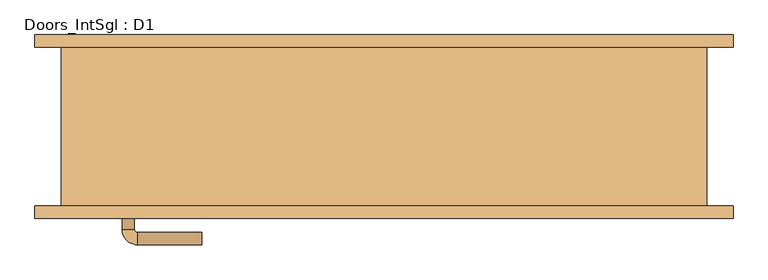
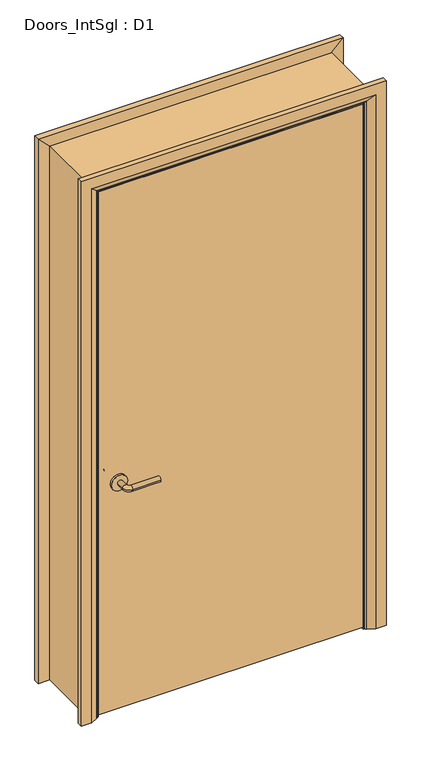
"""IFC4 building model written with IfcOpenShell, lengths in millimetres: door geometry, Doors_IntSgl : D1."""

from ifc_helpers import new_model, si_unit, point, frame, frame_2d, origin, place, context, project, spatial, polyline, circle_curve, ellipse_curve, trimmed, segment, composite_curve, outline, extrude, faceted_brep, source, transform, mapped, element, save
from ifc_brep_helpers import plane_surface, cylinder_surface, revolved_surface, advanced_brep


def doors_intsgl_d1_0a18db40(model_context):
    return source(origin(), model_context, "Body", "SolidModel", [
        advanced_brep(
        [(-426.4, -83.54, 900.0), (-406.4, -83.54, 900.0), (-426.4, -53.54, 900.0), (-406.4, -53.54, 900.0), (-401.4, -48.54, 900.0), (-401.4, -28.54, 900.0), (-296.4, -28.54, 900.0), (-296.4, -48.54, 900.0)],
        [
            (0, 1, circle_curve(frame((-416.4, -83.54, 900.0), z_axis=(0.0, -1.0, 0.0), x_axis=(1.0, 0.0, 0.0)), 10.0)),
            (1, 0, circle_curve(frame((-416.4, -83.54, 900.0), z_axis=(0.0, -1.0, 0.0), x_axis=(1.0, 0.0, 0.0)), 10.0)),
            (0, 2),
            (2, 3, circle_curve(frame((-416.4, -53.54, 900.0), z_axis=(0.0, -1.0, 0.0), x_axis=(1.0, 0.0, 0.0)), 10.0)),
            (3, 1),
            (3, 2, circle_curve(frame((-416.4, -53.54, 900.0), z_axis=(0.0, -1.0, 0.0), x_axis=(1.0, 0.0, 0.0)), 10.0)),
            (4, 3, circle_curve(frame((-401.4, -53.54, 900.0), z_axis=(0.0, 0.0, 1.0), x_axis=(-1.0, 0.0, 0.0)), 5.0)),
            (2, 5, circle_curve(frame((-401.4, -53.54, 900.0), z_axis=(0.0, 0.0, -1.0), x_axis=(-1.0, 0.0, 0.0)), 25.0)),
            (5, 4, circle_curve(frame((-401.4, -38.54, 900.0), z_axis=(-1.0, 0.0, 0.0), x_axis=(0.0, -1.0, 0.0)), 10.0)),
            (4, 5, circle_curve(frame((-401.4, -38.54, 900.0), z_axis=(-1.0, 0.0, 0.0), x_axis=(0.0, -1.0, 0.0)), 10.0)),
            (6, 7, circle_curve(frame((-296.4, -38.54, 900.0), z_axis=(1.0, 0.0, 0.0), x_axis=(0.0, -1.0, 0.0)), 10.0)),
            (7, 6, circle_curve(frame((-296.4, -38.54, 900.0), z_axis=(1.0, 0.0, 0.0), x_axis=(0.0, -1.0, 0.0)), 10.0)),
            (5, 6),
            (7, 4),
        ],
        [
            plane_surface(frame((-416.4, -83.54, 900.0), z_axis=(0.0, -1.0, 0.0), x_axis=(0.0, 0.0, 1.0))),
            cylinder_surface(frame((-416.4, -83.54, 900.0), z_axis=(0.0, -1.0, 0.0), x_axis=(1.0, 0.0, 0.0)), 10.0),
            revolved_surface(trimmed(ellipse_curve(frame((-416.4, -53.54, 900.0), z_axis=(0.0, -1.0, 0.0), x_axis=(1.0, 0.0, 0.0)), 10.0, 10.0), [point((-426.4, -53.54, 900.0))], [point((-406.4, -53.54, 900.0))], True, "CARTESIAN"), (-401.4, -53.54, 900.0), (0.0, 0.0, -1.0)),
            revolved_surface(trimmed(ellipse_curve(frame((-416.4, -53.54, 900.0), z_axis=(0.0, -1.0, 0.0), x_axis=(1.0, 0.0, 0.0)), 10.0, 10.0), [point((-406.4, -53.54, 900.0))], [point((-426.4, -53.54, 900.0))], True, "CARTESIAN"), (-401.4, -53.54, 900.0), (0.0, 0.0, -1.0)),
            plane_surface(frame((-296.4, -38.54, 900.0), z_axis=(1.0, 0.0, 0.0), x_axis=(0.0, 0.0, 1.0))),
            cylinder_surface(frame((-401.4, -38.54, 900.0), z_axis=(-1.0, 0.0, 0.0), x_axis=(0.0, -1.0, 0.0)), 10.0),
        ],
        [
            (0, [[1, 2]]),
            (1, [[-1, 3, 4, 5]]),
            (1, [[-2, -5, 6, -3]]),
            (2, [[7, -4, 8, 9]]),
            (3, [[-8, -6, -7, 10]]),
            (4, [[11, 12]]),
            (5, [[-9, 13, -12, 14]]),
            (5, [[-10, -14, -11, -13]]),
        ],
    ),
        extrude(outline(composite_curve([segment(trimmed(circle_curve(frame_2d((900.0, -418.9)), 30.0), [point((900.0, -448.9))], [point((900.0, -388.9))], False, "CARTESIAN"), True, "CONTINUOUS"), segment(trimmed(circle_curve(frame_2d((900.0, -418.9)), 30.0), [point((900.0, -388.9))], [point((900.0, -448.9))], False, "CARTESIAN"), True, "CONTINUOUS")], self_intersect=False)), frame((0.0, -91.54, 0.0), z_axis=(0.0, 1.0, 0.0), x_axis=(0.0, 0.0, 1.0)), (0.0, 0.0, 1.0), 8.0),
        advanced_brep(
        [(-426.4, -137.54, 900.0), (-406.4, -137.54, 900.0), (-406.4, -167.54, 900.0), (-426.4, -167.54, 900.0), (-401.4, -172.54, 900.0), (-401.4, -192.54, 900.0), (-296.4, -192.54, 900.0), (-296.4, -172.54, 900.0)],
        [
            (0, 1, circle_curve(frame((-416.4, -137.54, 900.0), z_axis=(0.0, 1.0, 0.0), x_axis=(1.0, 0.0, 0.0)), 10.0)),
            (1, 0, circle_curve(frame((-416.4, -137.54, 900.0), z_axis=(0.0, 1.0, 0.0), x_axis=(1.0, 0.0, 0.0)), 10.0)),
            (1, 2),
            (2, 3, circle_curve(frame((-416.4, -167.54, 900.0), z_axis=(0.0, 1.0, 0.0), x_axis=(1.0, 0.0, 0.0)), 10.0)),
            (3, 0),
            (3, 2, circle_curve(frame((-416.4, -167.54, 900.0), z_axis=(0.0, 1.0, 0.0), x_axis=(1.0, 0.0, 0.0)), 10.0)),
            (4, 5, circle_curve(frame((-401.4, -182.54, 900.0), z_axis=(-1.0, 0.0, 0.0), x_axis=(0.0, 1.0, 0.0)), 10.0)),
            (5, 3, circle_curve(frame((-401.4, -167.54, 900.0), z_axis=(0.0, 0.0, -1.0), x_axis=(-1.0, 0.0, 0.0)), 25.0)),
            (2, 4, circle_curve(frame((-401.4, -167.54, 900.0), z_axis=(0.0, 0.0, 1.0), x_axis=(-1.0, 0.0, 0.0)), 5.0)),
            (5, 4, circle_curve(frame((-401.4, -182.54, 900.0), z_axis=(-1.0, 0.0, 0.0), x_axis=(0.0, 1.0, 0.0)), 10.0)),
            (6, 7, circle_curve(frame((-296.4, -182.54, 900.0), z_axis=(1.0, 0.0, 0.0), x_axis=(0.0, 1.0, 0.0)), 10.0)),
            (7, 6, circle_curve(frame((-296.4, -182.54, 900.0), z_axis=(1.0, 0.0, 0.0), x_axis=(0.0, 1.0, 0.0)), 10.0)),
            (4, 7),
            (6, 5),
        ],
        [
            plane_surface(frame((-416.4, -137.54, 900.0), z_axis=(0.0, 1.0, 0.0), x_axis=(0.0, 0.0, 1.0))),
            cylinder_surface(frame((-416.4, -137.54, 900.0), z_axis=(0.0, 1.0, 0.0), x_axis=(1.0, 0.0, 0.0)), 10.0),
            revolved_surface(trimmed(ellipse_curve(frame((-416.4, -167.54, 900.0), z_axis=(0.0, -1.0, 0.0), x_axis=(1.0, 0.0, 0.0)), 10.0, 10.0), [point((-426.4, -167.54, 900.0))], [point((-406.4, -167.54, 900.0))], True, "CARTESIAN"), (-401.4, -167.54, 900.0), (0.0, 0.0, -1.0)),
            revolved_surface(trimmed(ellipse_curve(frame((-416.4, -167.54, 900.0), z_axis=(0.0, -1.0, 0.0), x_axis=(1.0, 0.0, 0.0)), 10.0, 10.0), [point((-406.4, -167.54, 900.0))], [point((-426.4, -167.54, 900.0))], True, "CARTESIAN"), (-401.4, -167.54, 900.0), (0.0, 0.0, -1.0)),
            plane_surface(frame((-296.4, -182.54, 900.0), z_axis=(1.0, 0.0, 0.0), x_axis=(0.0, 0.0, 1.0))),
            cylinder_surface(frame((-401.4, -182.54, 900.0), z_axis=(-1.0, 0.0, 0.0), x_axis=(0.0, 1.0, 0.0)), 10.0),
        ],
        [
            (0, [[1, 2]]),
            (1, [[3, 4, 5, -2]]),
            (1, [[-5, 6, -3, -1]]),
            (2, [[7, 8, -4, 9]]),
            (3, [[10, -9, -6, -8]]),
            (4, [[11, 12]]),
            (5, [[13, -11, 14, -7]]),
            (5, [[-14, -12, -13, -10]]),
        ],
    ),
        extrude(outline(composite_curve([segment(trimmed(circle_curve(frame_2d((900.0, -418.9)), 30.0), [point((900.0, -448.9))], [point((900.0, -388.9))], False, "CARTESIAN"), True, "CONTINUOUS"), segment(trimmed(circle_curve(frame_2d((900.0, -418.9)), 30.0), [point((900.0, -388.9))], [point((900.0, -448.9))], False, "CARTESIAN"), True, "CONTINUOUS")], self_intersect=False)), frame((0.0, -137.54, 0.0), z_axis=(0.0, 1.0, 0.0), x_axis=(0.0, 0.0, 1.0)), (0.0, 0.0, 1.0), 8.0),
        extrude(outline(polyline([(491.4, -91.54), (491.4, -129.54), (-491.4, -129.54), (-491.4, -91.54), (491.4, -91.54)])), frame((0.0, 0.0, 8.0), z_axis=(0.0, 0.0, 1.0), x_axis=(1.0, 0.0, 0.0)), (0.0, 0.0, 1.0), 2060.0),
        advanced_brep(
        [(568.4, -149.54, 0.0), (528.4, -149.54, 0.0), (502.4, -135.54, 0.0), (498.4, -129.54, 0.0), (568.4, -129.54, 0.0), (568.4, -129.54, 2145.0), (568.4, -149.54, 2145.0), (498.4, -129.54, 2075.0), (-498.4, -129.54, 2075.0), (-498.4, -129.54, 0.0), (-568.4, -129.54, 0.0), (-568.4, -129.54, 2145.0), (502.4, -135.54, 2079.0), (528.4, -149.54, 2105.0), (-568.4, -149.54, 2145.0), (-568.4, -149.54, 0.0), (-528.4, -149.54, 0.0), (-528.4, -149.54, 2105.0), (-502.4, -135.54, 0.0), (-502.4, -135.54, 2079.0)],
        [
            (0, 1),
            (1, 2),
            (2, 3, circle_curve(frame((506.4, -128.54, 0.0), z_axis=(0.0, 0.0, -1.0), x_axis=(1.0, 0.0, 0.0)), 8.0622577)),
            (3, 4),
            (4, 0),
            (4, 5),
            (5, 6),
            (6, 0),
            (3, 7),
            (7, 8),
            (8, 9),
            (9, 10),
            (10, 11),
            (11, 5),
            (2, 12),
            (12, 7, ellipse_curve(frame((506.4, -128.54, 2083.0), z_axis=(0.7071067811865475, 0.0, -0.7071067811865475), x_axis=(-0.7071067811865474, 0.0, -0.7071067811865476)), 11.4017543, 8.0622577)),
            (1, 13),
            (13, 12),
            (6, 14),
            (14, 15),
            (15, 16),
            (16, 17),
            (17, 13),
            (10, 15),
            (14, 11),
            (9, 18, circle_curve(frame((-506.4, -128.54, 0.0), z_axis=(0.0, 0.0, -1.0), x_axis=(-1.0, 0.0, 0.0)), 8.0622577)),
            (18, 16),
            (19, 18),
            (8, 19, ellipse_curve(frame((-506.4, -128.54, 2083.0), z_axis=(-0.7071067811865475, 0.0, -0.7071067811865475), x_axis=(-0.7071067811865474, 0.0, 0.7071067811865476)), 11.4017543, 8.0622577)),
            (19, 17),
            (12, 19),
        ],
        [
            plane_surface(frame((498.4, -129.54, 0.0), z_axis=(0.0, 0.0, -1.0), x_axis=(0.0, 1.0, 0.0))),
            plane_surface(frame((568.4, -149.54, 0.0), z_axis=(1.0, 0.0, 0.0), x_axis=(0.0, 0.0, 1.0))),
            plane_surface(frame((568.4, -129.54, 0.0), z_axis=(0.0, 1.0, 0.0), x_axis=(0.0, 0.0, 1.0))),
            cylinder_surface(frame((506.4, -128.54, 0.0), z_axis=(0.0, 0.0, -1.0), x_axis=(1.0, 0.0, 0.0)), 8.0622577),
            plane_surface(frame((502.4, -135.54, 0.0), z_axis=(-0.4740998230350126, -0.880471099922178, 0.0), x_axis=(0.0, 0.0, 1.0))),
            plane_surface(frame((528.4, -149.54, 0.0), z_axis=(0.0, -1.0, 0.0), x_axis=(0.0, 0.0, 1.0))),
            plane_surface(frame((-568.4, -149.54, 2145.0), z_axis=(-1.0, 0.0, 0.0), x_axis=(0.0, 0.0, -1.0))),
            plane_surface(frame((-498.4, -129.54, 0.0), z_axis=(0.0, 0.0, -1.0), x_axis=(0.0, 1.0, 0.0))),
            cylinder_surface(frame((-506.4, -128.54, 2075.0), z_axis=(0.0, 0.0, 1.0), x_axis=(-1.0, 0.0, 0.0)), 8.0622577),
            plane_surface(frame((-502.4, -135.54, 2079.0), z_axis=(0.47409982303501824, -0.8804710999221749, 0.0), x_axis=(0.0, 0.0, -1.0))),
            plane_surface(frame((568.4, -149.54, 2145.0), z_axis=(0.0, 0.0, 1.0), x_axis=(-1.0, 0.0, 0.0))),
            cylinder_surface(frame((498.4, -128.54, 2083.0), z_axis=(1.0, 0.0, 0.0), x_axis=(0.0, 0.0, 1.0)), 8.0622577),
            plane_surface(frame((502.4, -135.54, 2079.0), z_axis=(0.0, -0.8804710999221764, -0.4740998230350154), x_axis=(-1.0, 0.0, 0.0))),
        ],
        [
            (0, [[1, 2, 3, 4, 5]]),
            (1, [[6, 7, 8, -5]]),
            (2, [[9, 10, 11, 12, 13, 14, -6, -4]]),
            (3, [[15, 16, -9, -3]]),
            (4, [[17, 18, -15, -2]]),
            (5, [[-8, 19, 20, 21, 22, 23, -17, -1]]),
            (6, [[-13, 24, -20, 25]]),
            (7, [[-24, -12, 26, 27, -21]]),
            (8, [[28, -26, -11, 29]]),
            (9, [[-22, -27, -28, 30]]),
            (10, [[-14, -25, -19, -7]]),
            (11, [[31, -29, -10, -16]]),
            (12, [[-23, -30, -31, -18]]),
        ],
    ),
        extrude(outline(polyline([(0.0, -474.4), (2051.0, -474.4), (2051.0, 474.4), (0.0, 474.4), (0.0, 493.4), (2070.0, 493.4), (2070.0, -493.4), (0.0, -493.4), (0.0, -474.4)])), frame((0.0, -89.54, 0.0), z_axis=(0.0, 1.0, 0.0), x_axis=(0.0, 0.0, 1.0)), (0.0, 0.0, 1.0), 32.0),
        advanced_brep(
        [(-568.4, 149.54, 0.0), (-528.4, 149.54, 0.0), (-502.4, 135.54, 0.0), (-498.4, 129.54, 0.0), (-568.4, 129.54, 0.0), (-568.4, 129.54, 2145.0), (-568.4, 149.54, 2145.0), (-498.4, 129.54, 2075.0), (-502.4, 135.54, 2079.0), (-528.4, 149.54, 2105.0), (568.4, 149.54, 0.0), (568.4, 129.54, 0.0), (498.4, 129.54, 0.0), (502.4, 135.54, 0.0), (528.4, 149.54, 0.0), (568.4, 149.54, 2145.0), (528.4, 149.54, 2105.0), (502.4, 135.54, 2079.0), (498.4, 129.54, 2075.0), (568.4, 129.54, 2145.0)],
        [
            (0, 1),
            (1, 2),
            (2, 3, circle_curve(frame((-506.4, 128.54, 0.0), z_axis=(0.0, 0.0, -1.0), x_axis=(-1.0, 0.0, 0.0)), 8.0622577)),
            (3, 4),
            (4, 0),
            (4, 5),
            (5, 6),
            (6, 0),
            (3, 7),
            (7, 5),
            (2, 8),
            (8, 7, ellipse_curve(frame((-506.4, 128.54, 2083.0), z_axis=(-0.7071067811865475, 0.0, -0.7071067811865475), x_axis=(0.7071067811865474, 0.0, -0.7071067811865476)), 11.4017543, 8.0622577)),
            (1, 9),
            (9, 8),
            (6, 9),
            (10, 11),
            (11, 12),
            (12, 13, circle_curve(frame((506.4, 128.54, 0.0), z_axis=(0.0, 0.0, -1.0), x_axis=(1.0, 0.0, 0.0)), 8.0622577)),
            (13, 14),
            (14, 10),
            (15, 10),
            (14, 16),
            (16, 15),
            (13, 17),
            (17, 16),
            (12, 18),
            (18, 17, ellipse_curve(frame((506.4, 128.54, 2083.0), z_axis=(0.7071067811865475, 0.0, -0.7071067811865475), x_axis=(0.7071067811865474, 0.0, 0.7071067811865476)), 11.4017543, 8.0622577)),
            (11, 19),
            (19, 18),
            (15, 19),
            (5, 19),
            (15, 6),
            (7, 18),
            (8, 17),
            (9, 16),
        ],
        [
            plane_surface(frame((-498.4, 202.3410989, 0.0), z_axis=(0.0, 0.0, -1.0), x_axis=(1.0, 0.0, 0.0))),
            plane_surface(frame((-568.4, 149.54, 0.0), z_axis=(-1.0, 0.0, 0.0), x_axis=(0.0, 0.0, 1.0))),
            plane_surface(frame((-568.4, 129.54, 0.0), z_axis=(0.0, -1.0, 0.0), x_axis=(0.0, 0.0, 1.0))),
            cylinder_surface(frame((-506.4, 128.54, 0.0), z_axis=(0.0, 0.0, -1.0), x_axis=(-1.0, 0.0, 0.0)), 8.0622577),
            plane_surface(frame((-502.4, 135.54, 0.0), z_axis=(0.4740998230350183, 0.8804710999221749, 0.0), x_axis=(0.0, 0.0, 1.0))),
            plane_surface(frame((-528.4, 149.54, 0.0), z_axis=(0.0, 1.0, 0.0), x_axis=(0.0, 0.0, 1.0))),
            plane_surface(frame((498.4, 202.3410989, 0.0), z_axis=(0.0, 0.0, -1.0), x_axis=(-1.0, 0.0, 0.0))),
            plane_surface(frame((528.4, 149.54, 2105.0), z_axis=(0.0, 1.0, 0.0), x_axis=(0.0, 0.0, -1.0))),
            plane_surface(frame((502.4, 135.54, 2079.0), z_axis=(-0.4740998230350183, 0.8804710999221749, 0.0), x_axis=(0.0, 0.0, -1.0))),
            cylinder_surface(frame((506.4, 128.54, 2075.0), z_axis=(0.0, 0.0, 1.0), x_axis=(1.0, 0.0, 0.0)), 8.0622577),
            plane_surface(frame((568.4, 129.54, 2145.0), z_axis=(0.0, -1.0, 0.0), x_axis=(0.0, 0.0, -1.0))),
            plane_surface(frame((568.4, 149.54, 2145.0), z_axis=(1.0, 0.0, 0.0), x_axis=(0.0, 0.0, -1.0))),
            plane_surface(frame((-568.4, 149.54, 2145.0), z_axis=(0.0, 0.0, 1.0), x_axis=(1.0, 0.0, 0.0))),
            plane_surface(frame((-568.4, 129.54, 2145.0), z_axis=(0.0, -1.0, 0.0), x_axis=(1.0, 0.0, 0.0))),
            cylinder_surface(frame((-498.4, 128.54, 2083.0), z_axis=(-1.0, 0.0, 0.0), x_axis=(0.0, 0.0, 1.0)), 8.0622577),
            plane_surface(frame((-502.4, 135.54, 2079.0), z_axis=(0.0, 0.8804710999221749, -0.4740998230350183), x_axis=(1.0, 0.0, 0.0))),
            plane_surface(frame((-528.4, 149.54, 2105.0), z_axis=(0.0, 1.0, 0.0), x_axis=(1.0, 0.0, 0.0))),
        ],
        [
            (0, [[1, 2, 3, 4, 5]]),
            (1, [[6, 7, 8, -5]]),
            (2, [[9, 10, -6, -4]]),
            (3, [[11, 12, -9, -3]]),
            (4, [[13, 14, -11, -2]]),
            (5, [[-8, 15, -13, -1]]),
            (6, [[16, 17, 18, 19, 20]]),
            (7, [[21, -20, 22, 23]]),
            (8, [[-22, -19, 24, 25]]),
            (9, [[-24, -18, 26, 27]]),
            (10, [[-26, -17, 28, 29]]),
            (11, [[-28, -16, -21, 30]]),
            (12, [[31, -30, 32, -7]]),
            (13, [[33, -29, -31, -10]]),
            (14, [[34, -27, -33, -12]]),
            (15, [[35, -25, -34, -14]]),
            (16, [[-32, -23, -35, -15]]),
        ],
    ),
        faceted_brep([(-493.4, -129.54, 0.0), (-525.4, -129.54, 0.0), (-525.4, 129.54, 0.0), (-493.4, 129.54, 0.0), (-493.4, 129.54, 2070.0), (-493.4, -129.54, 2070.0), (-525.4, 129.54, 2102.0), (-525.4, -129.54, 2102.0), (493.4, -129.54, 0.0), (493.4, 129.54, 0.0), (525.4, 129.54, 0.0), (525.4, -129.54, 0.0), (493.4, -129.54, 2070.0), (525.4, -129.54, 2102.0), (525.4, 129.54, 2102.0), (493.4, 129.54, 2070.0)], [[[0, 1, 2, 3]], [[3, 4, 5, 0]], [[2, 6, 4, 3]], [[1, 7, 6, 2]], [[0, 5, 7, 1]], [[8, 9, 10, 11]], [[12, 8, 11, 13]], [[13, 11, 10, 14]], [[14, 10, 9, 15]], [[15, 9, 8, 12]], [[4, 15, 12, 5]], [[6, 14, 15, 4]], [[7, 13, 14, 6]], [[5, 12, 13, 7]]]),
    ])


if __name__ == "__main__":
    model = new_model("IFC4")
    model_context = context("Model", 3, world=origin())
    ifc_project = project(units=[si_unit("LENGTHUNIT", "METRE", prefix="MILLI")], contexts=[model_context])
    site = spatial("IfcSite", under=ifc_project)
    building = spatial("IfcBuilding", under=site)
    placement = place(None, origin())
    doors_intsgl_d1_shape = doors_intsgl_d1_0a18db40(model_context)
    element("IfcDoor", 1, ObjectType="Doors_IntSgl : D1", at=placement, inside=building, context=model_context, shape_type="MappedRepresentation", body=[
        mapped(doors_intsgl_d1_shape, transform((0.0, 0.0, 0.0), x_axis=(1.0, 0.0, 0.0), y_axis=(0.0, 1.0, 0.0), z_axis=(0.0, 0.0, 1.0))),
    ])
    save(model, "model.ifc")

# Revit data of these elements
# Type "Doors_IntSgl : D1"
#   Type Mark = "46"
#   Type Comments = "Internal Single"
#   Operation = "SingleSwingRight"
#   Manufacturer = "Revit"
#   Keynote = "L20"
#   Description = "Internal Single Door"
#   Analytic Construction = "Metal"
#   UnderCut = 0.026247 ft
#   Tolerance = 0.006562 ft
#   Thickness = 0.124672 ft
#   Thermal Resistance (R) = 0.270117 (m²·K)/W
#   Structural Tolerance = 0.026247 ft
#   StopDepth = 0.104987 ft
#   Stop Thickness = 0.062336 ft
#   Rough Width = 3.5 ft
#   Rough Height = 6.922572 ft
#   Height to Top Lock Rail = 3.28084 ft
#   Heat Transfer Coefficient (U) = 3.7021 W/(m²·K)
#   Handle Z Distance = 2.952756 ft
#   Handle X Distance = 0.246063 ft
#   Frame Thickness = 0.104987 ft
#   Door Panel Width = 3.224409 ft
#   Door Panel Thickness = 0.124672 ft
#   Door Panel Offset = 0.0 ft
#   Height = 6.922572 ft
#   Width = 3.5 ft
#   Door Panel Height = 6.75853 ft
#   Architrave Setback = 0.016404 ft
#   Vis - Ironmongery = yes
#   Material Ironmongery = Door - Handle
#   Material Frame = Door - Frame/Mullion (1)
#   Material Door = Door - Panel
#   Material Architrave = Door - Architrave
#   Visual Light Transmittance = 0
#   Solar Heat Gain Coefficient = 0
#   Function = (empty or 0)
#   Wall Closure = (empty or 0)
# Element 1 (IfcDoor, "Doors_IntSgl : D1")
#   Materials on its faces: "Door - Architrave", "Door - Handle", "Door - Frame/Mullion (1)", "Door - Panel"
# Materials
#   "Door - Handle": colour RGB 0 0 0, transparency 0, Keynote = "P21", Cost = 0
#   "Door - Frame/Mullion (1)": class "Wood", colour RGB 212 179 113, transparency 0, Keynote = "L20", Cost = 0
#   "Door - Panel": class "Wood", colour RGB 210 159 95, transparency 0, Keynote = "L20", Cost = 0
#   "Door - Architrave": class "Wood", colour RGB 154 90 5, transparency 0, Keynote = "P20", Cost = 0
